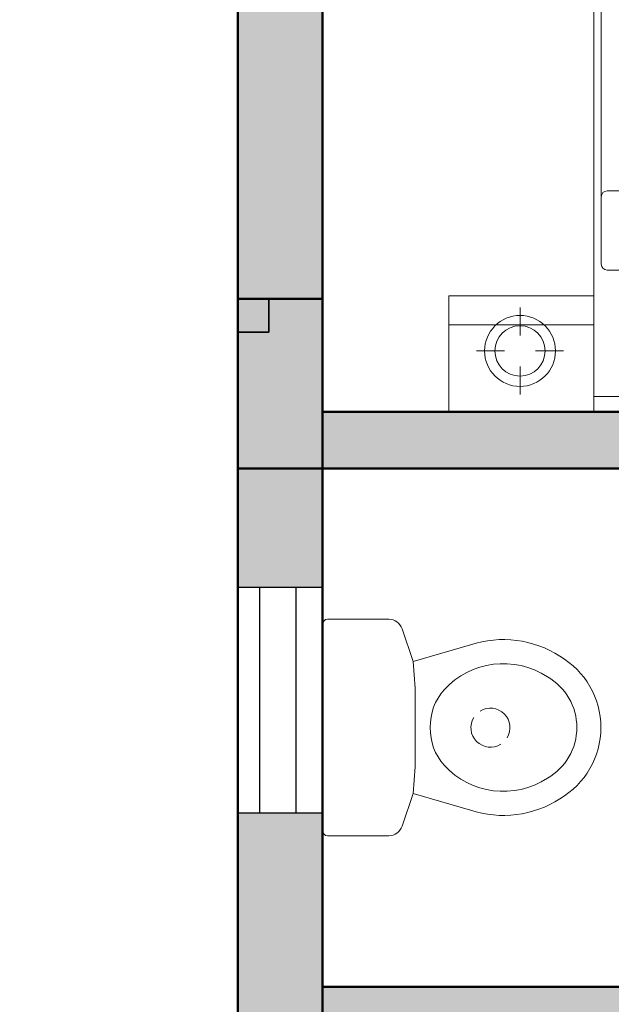
# Model space of a CAD drawing. Units: inches. Extents: x -7 to 1228, y -146 to 1091.
# Tile 71 of 88: x 611 to 674, y 785 to 890. Entities that reach past the tile are written whole.
import ezdxf

# ---------------------------------------------------------------- set-up
doc = ezdxf.new("R2010")
doc.units = ezdxf.units.IN
for name, color, linetype, lineweight in [('A-COLS', 6, 'Continuous', 35), ('A-FLOR-FIXT', 8, 'Continuous', 18), ('A-FURN', 8, 'Continuous', 18), ('A-GLAZ', 175, 'Continuous', 25), ('A-WALL', 7, 'Continuous', 50), ('A-WALL-PATT', 251, 'Continuous', 13)]:
    doc.layers.add(name, color=color, linetype=linetype, lineweight=lineweight)
doc.styles.add('DIM_FONT', font='SIMPLEX.shx', dxfattribs={"width": 0.8})

# ---------------------------------------------------------------- blocks, each defined once
blk = doc.blocks.new('A$C4F634EDD')
for p, q in [((0, 2.6295), (0, 2.2295)), ((0.5, 2.6295), (0, 2.6295)), ((0.5, 2.6295), (2.3, 2.6295)), ((0.5, 0.5295), (0.5, 2.6295)), ((0.5, 2.2295), (0.5, 2.6295)), ((0.2457, 2.5697), (0.2457, 2.4733)), ((0.5, 2.5771), (2.3, 2.5771)), ((0.0957, 2.4197), (0.192, 2.4197)), ((0.2994, 2.4197), (0.3957, 2.4197)), ((0.2457, 2.366), (0.2457, 2.2697)), ((0, 2.3301), (0.5, 2.3301)), ((0, 2.2295), (0.5, 2.2295)), ((1.5035, 2.141), (0.5458, 2.141)), ((0.5258, 2.121), (0.5258, 0.5617)), ((0.5458, 1.8684), (1.5653, 1.8684))]:
    blk.add_line(p, q)
for radius in [0.1222, 0.0865]:
    blk.add_circle((0.2457, 2.4197), radius)
for centre, start, end in [((0.5458, 2.121), 90, 180), ((0.5458, 1.8884), 180, 270)]:
    blk.add_arc(centre, 0.02, start, end)
at = {"style": 'DIM_FONT', "width": 0.8, "flags": 9}
for tag, p in [('YSIZE', (0.5, 2.6295)), ('XSIZE', (0.5, 2.6295)), ('XSIZE', (2.2985, 2.6295)), ('YSIZE', (2.2985, 2.6295))]:
    blk.add_attdef(tag, p, '', height=0.0005, dxfattribs=at)
blk = doc.blocks.new('A$C7B5C7CD4')
at = {"ltscale": 20}
for p, q in [((0.243, 0.625), (0.011, 0.625)), ((0.243, 0.625), (0.475, 0.625)), ((0, 0.614), (0, 0.4765)), ((0.486, 0.614), (0.486, 0.4765)), ((0.0212, 0.4467), (0.0946, 0.4214)), ((0.4648, 0.4467), (0.3914, 0.4214)), ((0.0946, 0.4214), (0.0576, 0.293)), ((0.0946, 0.4214), (0.1544, 0.4173)), ((0.3914, 0.4214), (0.3316, 0.4173)), ((0.3914, 0.4214), (0.4284, 0.293)), ((0.3316, 0.4173), (0.1544, 0.4173))]:
    blk.add_line(p, q, dxfattribs=at)
for centre, radius, start, end in [((0.011, 0.614), 0.011, 90, 180), ((0.475, 0.614), 0.011, 0, 90), ((0.0315, 0.4765), 0.0315, 180, 251), ((0.4545, 0.4765), 0.0315, 289, 0), ((0.24, 0.2602), 0.123, 88.6158, 131.7414), ((0.246, 0.2602), 0.123, 48.2586, 91.3842), ((0.2796, 0.219), 0.18, 132.4207, 213.289), ((0.2064, 0.219), 0.18, 326.711, 47.5793), ((0.2796, 0.219), 0.234, 161.5846, 212.8753), ((0.2064, 0.219), 0.234, 327.1247, 18.4154), ((0.243, 0.185), 0.131, 209.6292, 270), ((0.243, 0.185), 0.131, 270, 330.3708), ((0.243, 0.185), 0.185, 210.1745, 270), ((0.243, 0.185), 0.185, 270, 329.8255)]:
    blk.add_arc(centre, radius, start, end, dxfattribs=at)
for start, end in [(58.1785, 211.8215), (238.1785, 31.8215)]:
    blk.add_arc((0.2426, 0.2481), 0.0439, start, end)
blk = doc.blocks.new('WIN-24')
for p, q in [((0, 0), (0, 24)), ((0, 24), (9, 24)), ((2.34, 0), (2.34, 24)), ((2.34, 24), (6.14, 24)), ((6.14, 24), (6.14, 0)), ((9, 24), (9, 0)), ((9, 0), (0, 0))]:
    blk.add_line(p, q)

msp = doc.modelspace()

# ---------------------------------------------------------------- hatches: boundary and pattern name
at = {"layer": 'A-COLS'}
h = msp.add_hatch(color=256, dxfattribs=at)
h.dxf.hatch_style = 1
h.paths.add_polyline_path([(634, 842), (643, 842), (643, 860), (637.29, 860), (637.29, 856.45), (634, 856.45)])
h = msp.add_hatch(color=256, dxfattribs=at)
h.dxf.hatch_style = 1
h.paths.add_polyline_path([(637.29, 856.45), (637.29, 860), (634, 860), (634, 856.45)])
at = {"layer": 'A-WALL-PATT'}
h = msp.add_hatch(color=256, dxfattribs=at)
h.dxf.hatch_style = 1
h.paths.add_polyline_path([(69, 568), (60, 568), (60, 493), (63.29, 493), (69, 493)])
h.paths.add_polyline_path([(69, 662.41), (60, 662.41), (60, 586), (69, 586)], flags=17)
h.paths.add_polyline_path([(69, 723), (184, 723), (184, 734), (179, 734), (179, 728), (69, 728), (69, 741.62), (60, 741.62), (60, 698.41), (69, 698.41)], flags=17)
h.paths.add_polyline_path([(69, 782), (231, 782), (231, 728), (231, 723), (231, 586), (236, 586), (236, 787), (69, 787), (69, 800.13), (60, 800.13), (60, 765.62), (69, 765.62)])
h.paths.add_polyline_path([(184, 842), (189, 842), (189, 848), (173, 848), (173, 842), (179, 842), (179, 787), (184, 787)])
h.paths.add_polyline_path([(118.22, 69), (69, 69), (69, 60), (118.22, 60)])
h.paths.add_polyline_path([(227, 69), (154.22, 69), (154.22, 60), (227, 60)])
h.paths.add_polyline_path([(236, 60), (232.71, 60), (227, 60), (227, 36), (236, 36)])
h.paths.add_polyline_path([(389, 60), (380, 60), (380, 36), (389, 36)])
h.paths.add_polyline_path([(384, 181), (380, 181), (380, 115), (380, 78), (384, 78)])
h.paths.add_polyline_path([(380, 115), (334.55, 115), (334.55, 109), (380, 109)])
h.paths.add_polyline_path([(274.55, 115), (236, 115), (236, 201), (232.71, 201), (231, 201), (231, 78), (236, 78), (236, 109), (274.55, 109)])
h.paths.add_polyline_path([(69, 123), (60, 123), (60, 78), (69, 78)])
h.paths.add_polyline_path([(69, 201), (60, 201), (60, 159), (69, 159)])
h.paths.add_polyline_path([(143, 219), (69, 219), (69, 213), (143, 213)], flags=17)
h.paths.add_polyline_path([(189, 219), (184, 219), (184, 274), (231, 274), (231, 219), (236, 219), (236, 279), (184, 279), (184, 297), (179, 297), (179, 279), (69, 279), (69, 290.91), (60, 290.91), (60, 262.18), (69, 262.18), (69, 274), (179, 274), (179, 219), (173, 219), (173, 213), (189, 213)])
h.paths.add_polyline_path([(69, 238.18), (60, 238.18), (60, 219), (69, 219)], flags=17)
h.paths.add_polyline_path([(69, 333), (60, 333), (60, 314.91), (69, 314.91), (69, 316.96)])
h.paths.add_polyline_path([(190, 338), (184, 338), (69, 338), (69, 333), (179, 333), (179, 327), (184, 327), (184, 333.02), (190, 333.05)])
h.paths.add_polyline_path([(69, 386.81), (60, 386.81), (60, 351), (69, 351)])
h.paths.add_polyline_path([(69, 475), (60, 475), (60, 422.81), (69, 422.81)])
h.paths.add_polyline_path([(236, 475), (231, 475), (231, 351.24), (236, 351.24)])
h.paths.add_polyline_path([(384, 475), (380, 475), (380, 362), (384, 362)])
h.paths.add_polyline_path([(547, 307), (439, 307), (439, 356), (445, 356), (445, 362), (433, 362), (433, 307), (380, 307), (380, 244), (380, 241), (384, 241), (384, 301), (433, 301), (433, 277), (439, 277), (439, 301), (547, 301)])
h.paths.add_polyline_path([(547, 241), (439, 241), (439, 247), (433, 247), (433, 235), (547, 235)])
h.paths.add_polyline_path([(450, 69), (440.29, 69), (424.89, 69), (389, 69), (389, 60), (450, 60)])
h.paths.add_polyline_path([(547, 69), (486, 69), (486, 60), (547, 60)])
h.paths.add_polyline_path([(556, 148.27), (547, 148.27), (547, 78), (556, 78)])
h.paths.add_polyline_path([(556, 223), (547, 223), (547, 195), (547, 184.27), (556, 184.27)])
h.paths.add_polyline_path([(556, 311.19), (547, 311.19), (547, 273.08), (556, 273.08)])
h.paths.add_polyline_path([(556, 344), (552.71, 344), (547, 344), (547, 335.19), (556, 335.19)])
h.paths.add_polyline_path([(556, 249.08), (547, 249.08), (547, 241), (556, 241)])
h.paths.add_polyline_path([(547, 362), (475, 362), (475, 356), (547, 356)], flags=0)
h.paths.add_polyline_path([(556, 399.62), (547, 399.62), (547, 362), (556, 362)])
h.paths.add_polyline_path([(556, 475), (547, 475), (547, 435.62), (556, 435.62)])
h.paths.add_polyline_path([(547, 493), (389, 493), (389, 487), (547, 487)])
h.paths.add_polyline_path([(380, 493), (278, 493), (278, 487), (380, 487)])
h.paths.add_polyline_path([(227, 493), (69, 493), (69, 487), (227, 487)])
h.paths.add_polyline_path([(643, 122.44), (634, 122.44), (634, 78), (643, 78)])
h.paths.add_polyline_path([(702.5, 69), (692.79, 69), (677.39, 69), (643, 69), (643, 60), (702.5, 60)])
h.paths.add_polyline_path([(798, 69), (738.5, 69), (738.5, 60), (798, 60)])
h.paths.add_polyline_path([(807, 60), (803.71, 60), (798, 60), (798, 36), (807, 36)])
h.paths.add_polyline_path([(807, 109), (846.75, 109), (846.75, 115), (807, 115), (807, 159), (802, 159), (802, 78), (807, 78)])
h.paths.add_polyline_path([(807, 201), (802, 201), (802, 195), (807, 195)])
h.paths.add_polyline_path([(643, 201), (634, 201), (634, 158.44), (643, 158.44)])
h.paths.add_polyline_path([(756, 225), (751, 225), (751, 219), (643, 219), (643, 213), (756, 213)])
h.paths.add_polyline_path([(643, 240.85), (634, 240.85), (634, 219), (643, 219)])
h.paths.add_polyline_path([(643, 274), (643, 288.63), (634, 288.63), (634, 264.85), (643, 264.85)])
h.paths.add_polyline_path([(802, 279), (756, 279), (756, 297), (751, 297), (751, 279), (643, 279), (643, 274), (751, 274), (751, 255), (756, 255), (756, 274), (802, 274)])
h.paths.add_polyline_path([(807, 333), (803.71, 333), (802, 333), (802, 279), (802, 274), (802, 219), (807, 219)])
h.paths.add_polyline_path([(956, 182), (951, 182), (951, 115), (906.75, 115), (906.75, 109), (951, 109), (951, 78), (956, 78)])
h.paths.add_polyline_path([(960, 60), (951, 60), (951, 36), (960, 36)])
h.paths.add_polyline_path([(1021, 69), (1005.78, 69), (960, 69), (960, 60), (1021, 60)])
h.paths.add_polyline_path([(956, 224), (951, 224), (951, 218), (956, 218)])
h.paths.add_polyline_path([(956, 302), (1004, 302), (1004, 278), (1010, 278), (1010, 302), (1118, 302), (1118, 290.81), (1127, 290.81), (1127, 326.97), (1118, 326.97), (1118, 320.97), (1118, 307), (1010, 307), (1010, 356), (1016, 356), (1016, 362), (1004, 362), (1004, 307), (951, 307), (951, 244), (951, 242), (954.29, 242), (956, 242)])
h.paths.add_polyline_path([(643, 333), (634, 333), (634, 312.63), (643, 312.63), (643, 316.96)])
h.paths.add_polyline_path([(756, 338), (643, 338), (643, 333), (751, 333), (751, 327), (756, 327)])
h.paths.add_polyline_path([(643, 388), (634, 388), (634, 351), (643, 351)])
h.paths.add_polyline_path([(807, 357), (802, 357), (802, 351), (807, 351)])
h.paths.add_polyline_path([(807, 475), (802, 475), (802, 393), (807, 393)])
h.paths.add_polyline_path([(643, 475), (634, 475), (634, 424), (643, 424)])
h.paths.add_polyline_path([(798, 493), (643, 493), (643, 487), (798, 487)])
h.paths.add_polyline_path([(634, 493), (556, 493), (556, 487), (634, 487)])
h.paths.add_polyline_path([(813, 493), (807, 493), (807, 487), (813, 487)])
h.paths.add_polyline_path([(951, 493), (849, 493), (849, 487), (951, 487)])
h.paths.add_polyline_path([(956, 484), (951, 484), (951, 374), (956, 374)])
h.paths.add_polyline_path([(1109, 493), (969, 493), (969, 487), (1109, 487)])
h.paths.add_polyline_path([(1127, 484), (1118, 484), (1118, 450.64), (1127, 450.64)])
h.paths.add_polyline_path([(1127, 414.64), (1118, 414.64), (1118, 365), (1127, 365)])
h.paths.add_polyline_path([(1109, 362), (1046, 362), (1046, 356), (1109, 356)], flags=17)
h.paths.add_polyline_path([(1127, 356), (1123.45, 356), (1118, 356), (1118, 350.97), (1127, 350.97)], flags=0)
h.paths.add_polyline_path([(1127, 266.81), (1118, 266.81), (1118, 262.36), (1118, 242), (1127, 242)], flags=17)
h.paths.add_polyline_path([(1118, 242), (1010, 242), (1010, 248), (1004, 248), (1004, 237), (1118, 237)])
h.paths.add_polyline_path([(1127, 224), (1118, 224), (1118, 170), (1127, 170)])
h.paths.add_polyline_path([(1127, 134), (1118, 134), (1118, 78), (1127, 78)])
h.paths.add_polyline_path([(1118, 69), (1057, 69), (1057, 60), (1118, 60)])
h.paths.add_polyline_path([(227, 571.55), (227, 574), (69, 574), (69, 568), (227, 568)])
h.paths.add_polyline_path([(380, 571.55), (380, 574), (278, 574), (278, 568), (380, 568)])
h.paths.add_polyline_path([(242, 574), (236, 574), (236, 568), (242, 568)])
h.paths.add_polyline_path([(547, 571.55), (547, 574), (389, 574), (389, 568), (547, 568)])
h.paths.add_polyline_path([(384, 733), (380, 733), (380, 586), (384, 586)])
h.paths.add_polyline_path([(556, 646), (634, 646), (634, 655), (547, 655), (547, 586), (556, 586)])
h.paths.add_polyline_path([(634, 574), (556, 574), (556, 568), (634, 568)])
h.paths.add_polyline_path([(643, 655), (634, 655), (634, 586), (643, 586)])
h.paths.add_polyline_path([(798, 574), (643, 574), (643, 568), (798, 568)])
h.paths.add_polyline_path([(643, 663.85), (634, 663.85), (634, 655), (643, 655)])
h.paths.add_polyline_path([(556, 676.97), (547, 676.97), (547, 655), (556, 655)])
h.paths.add_polyline_path([(556, 733), (547, 733), (547, 712.97), (556, 712.97)])
h.paths.add_polyline_path([(643, 710), (634, 710), (634, 699.85), (643, 699.85)])
h.paths.add_polyline_path([(807, 668), (802, 668), (802, 586), (807, 586)])
h.paths.add_polyline_path([(951, 574), (849, 574), (849, 568), (951, 568)])
h.paths.add_polyline_path([(956, 691), (951, 691), (951, 577), (956, 577)])
h.paths.add_polyline_path([(1109, 574), (969, 574), (969, 568), (1109, 568)])
h.paths.add_polyline_path([(1127, 643.4), (1118, 643.4), (1118, 577), (1127, 577)])
h.paths.add_polyline_path([(1127, 568), (1123.45, 568), (1118, 568), (1118, 493), (1127, 493)])
h.paths.add_polyline_path([(1127, 733), (1118, 733), (1118, 679.4), (1127, 679.4)])
h.paths.add_polyline_path([(1127, 777.35), (1118, 777.35), (1118, 770.04), (1118, 751), (1127, 751)], flags=17)
h.paths.add_polyline_path([(1118, 751), (1010, 751), (1010, 757), (1004, 757), (1004, 745), (1118, 745)])
h.paths.add_polyline_path([(956, 811), (1004, 811), (1004, 787), (1010, 787), (1010, 811), (1017.87, 811), (1017.87, 811.63, -0.414214), (1018.25, 812), (1031.98, 812, -0.414214), (1032.35, 811.63), (1032.35, 811), (1118, 811), (1118, 801.35), (1127, 801.35), (1127, 834.69), (1118, 834.69), (1118, 830.24), (1118, 817), (1010, 817), (1010, 866), (1016, 866), (1016, 872), (1004, 872), (1004, 817), (956, 817), (956, 866), (951, 866), (951, 751), (954.29, 751), (956, 751)])
h.paths.add_polyline_path([(1118, 872), (1046, 872), (1046, 866), (1118, 866)], flags=17)
h.paths.add_polyline_path([(1127, 924.71), (1118, 924.71), (1118, 884), (1127, 884)])
h.paths.add_polyline_path([(1127, 866), (1123.71, 866), (1118, 866), (1118, 858.69), (1127, 858.69)], flags=17)
h.paths.add_polyline_path([(956, 983), (951, 983), (951, 952), (807, 952), (807, 983), (802, 983), (802, 902), (807, 902), (807, 946), (951, 946), (951, 884), (956, 884)])
h.paths.add_polyline_path([(807, 842), (802, 842), (802, 787), (756, 787), (756, 806), (751, 806), (751, 787), (643, 787), (643, 782), (751, 782), (751, 764), (756, 764), (756, 782), (802, 782), (802, 728), (807, 728)])
h.paths.add_polyline_path([(756, 848), (643, 848), (643, 842), (751, 842), (751, 836), (756, 836)])
h.paths.add_polyline_path([(756, 734), (751, 734), (751, 728), (643, 728), (643, 723), (756, 723)])
h.paths.add_polyline_path([(643, 749.79), (634, 749.79), (634, 728), (637.29, 728), (643, 728)])
h.paths.add_polyline_path([(643, 805.41), (634, 805.41), (634, 773.79), (643, 773.79)])
h.paths.add_polyline_path([(643, 896.66), (634, 896.66), (634, 860), (637.29, 860), (643, 860)])
h.paths.add_polyline_path([(643, 842), (634, 842), (634, 829.41), (643, 829.41)])
h.paths.add_polyline_path([(643, 983), (634, 983), (634, 932.66), (643, 932.66)])
h.paths.add_polyline_path([(1127, 983), (1118, 983), (1118, 960.71), (1127, 960.71)])
h.paths.add_polyline_path([(1118, 1001), (1077.53, 1001), (1077.53, 992), (1118, 992)])
h.paths.add_polyline_path([(1041.53, 1001), (960, 1001), (960, 992), (1041.53, 992)])
h.paths.add_polyline_path([(960, 1025), (951, 1025), (951, 1001), (954.29, 1001), (960, 1001)])
h.paths.add_polyline_path([(807, 1025), (798, 1025), (798, 1001), (807, 1001)])
h.paths.add_polyline_path([(798, 1001), (738.5, 1001), (738.5, 992), (798, 992)])
h.paths.add_polyline_path([(702.5, 1001), (643, 1001), (643, 992), (702.5, 992)])
h.paths.add_polyline_path([(547, 1001), (499.11, 1001), (499.11, 992), (547, 992)])
h.paths.add_polyline_path([(463.11, 1001), (389, 1001), (389, 992), (463.11, 992)])
h.paths.add_polyline_path([(389, 1025), (380, 1025), (380, 1022), (380, 1001), (383.29, 1001), (389, 1001)])
h.paths.add_polyline_path([(236, 1025), (227, 1025), (227, 1001), (236, 1001)])
h.paths.add_polyline_path([(236, 983), (231, 983), (231, 860), (236, 860)])
h.paths.add_polyline_path([(274.55, 952), (236, 952), (236, 946), (274.55, 946)])
h.paths.add_polyline_path([(380, 952), (334.55, 952), (334.55, 946), (380, 946)])
h.paths.add_polyline_path([(384, 983), (380, 983), (380, 884), (383.29, 884), (384, 884)])
h.paths.add_polyline_path([(227, 1001), (155.01, 1001), (155.01, 992), (162.87, 992), (227, 992)])
h.paths.add_polyline_path([(119.01, 1001), (69, 1001), (69, 992), (119.01, 992)])
h.paths.add_polyline_path([(69, 983), (60, 983), (60, 922.99), (69, 922.99)])
h.paths.add_polyline_path([(69, 886.99), (60, 886.99), (60, 860), (63.29, 860), (69, 860)])
h.paths.add_polyline_path([(143, 848), (69, 848), (69, 842), (143, 842)])

# ---------------------------------------------------------------- linework, layer by layer
at = {"layer": 'A-COLS'}
msp.add_lwpolyline([(634, 860), (637.29, 860), (637.29, 856.45), (634, 856.45)], close=True, dxfattribs=at)
at = {"layer": 'A-WALL'}
for p, q in [((634, 1001), (634, 655)), ((634, 568), (634, 1001)), ((643, 1001), (643, 848)), ((643, 568), (643, 1001)), ((634, 860), (643, 860)), ((634, 842), (634, 860)), ((643, 860), (643, 842)), ((643, 842), (643, 848)), ((756, 848), (643, 848)), ((643, 842), (634, 842)), ((643, 842), (643, 787)), ((751, 842), (643, 842)), ((751, 787), (643, 787))]:
    msp.add_line(p, q, dxfattribs=at)

# ---------------------------------------------------------------- block references
at = {"layer": 'A-FLOR-FIXT', "xscale": 47.26153857112405, "yscale": 47.26153857112405, "zscale": 47.26153857112405, "rotation": 90}
msp.add_blockref('A$C7B5C7CD4', (672.54, 803.02), dxfattribs=at)
at = {"layer": 'A-FURN', "xscale": -30.79356024027943, "yscale": 30.79356024027943, "zscale": 30.79356024027943, "rotation": 180}
msp.add_blockref('A$C4F634EDD', (656.39, 928.97), dxfattribs=at)
at = {"layer": 'A-GLAZ'}
msp.add_blockref('WIN-24', (634, 805.4), dxfattribs=at)

doc.saveas('drawing.dxf')
